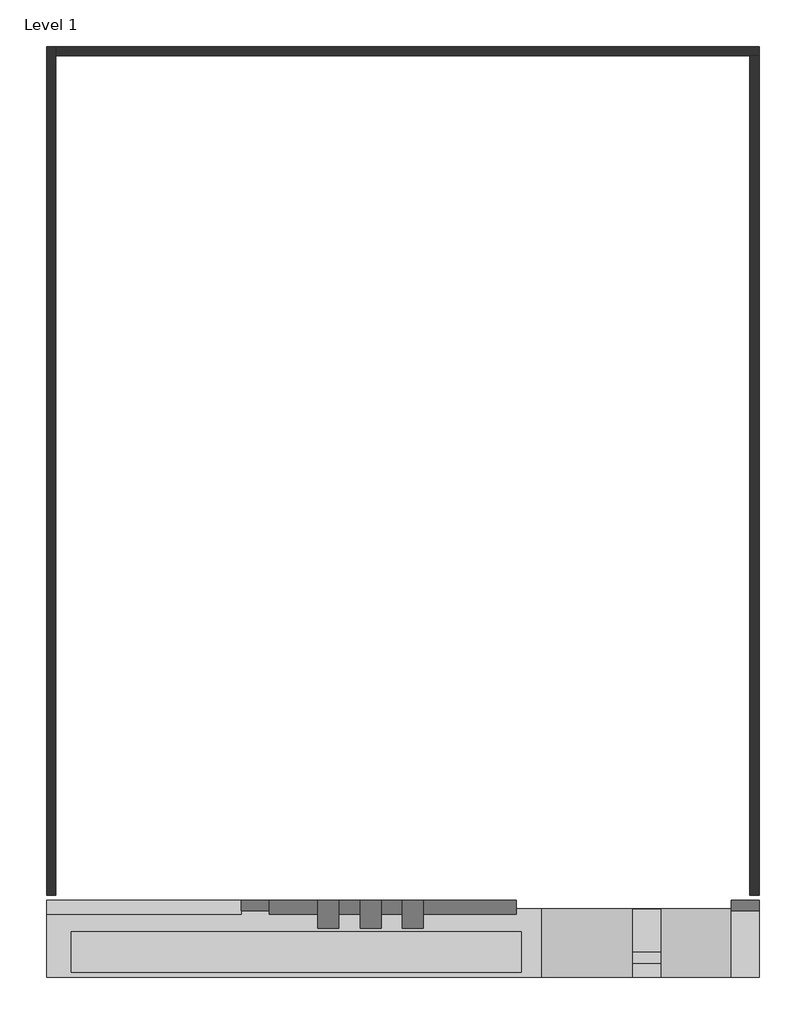
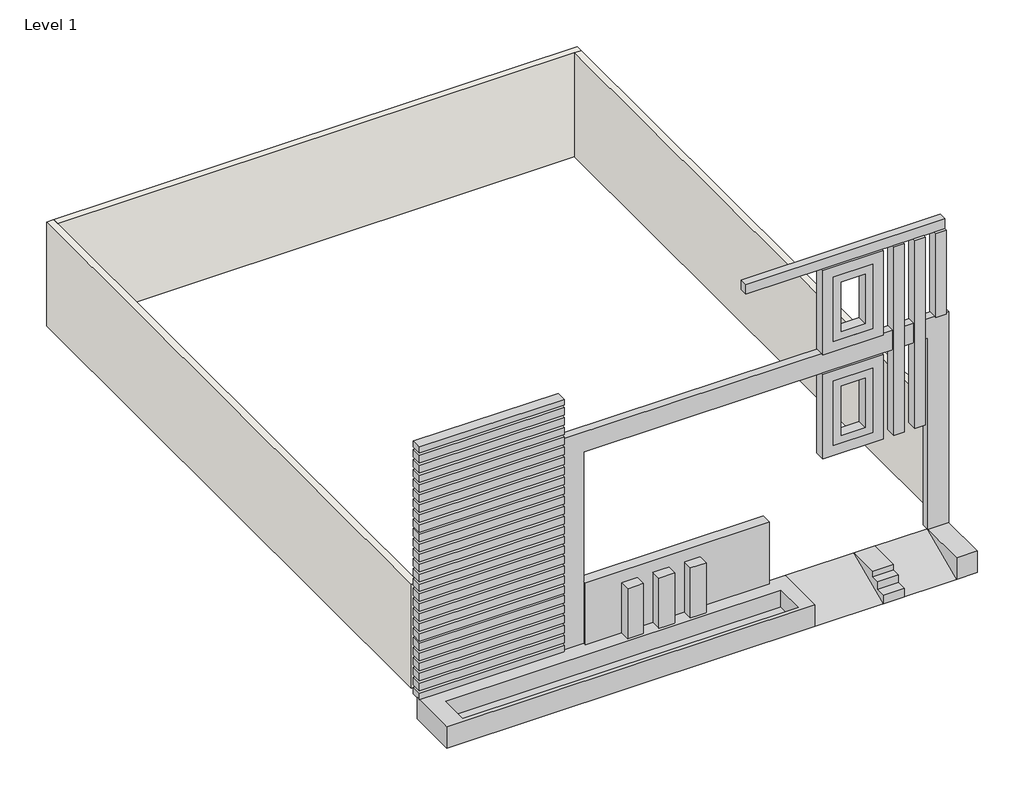
# One storey: 3 walls, 1 proxy.
"""IFC4 building model written with IfcOpenShell, lengths in millimetres."""

from ifc_helpers import new_model, si_unit, frame, origin, place, context, project, spatial, polyline, outline, extrude, faceted_brep, transform, mapped, element, save
from components import electrical_fixtures_1_electrical_fixtures_1_7c594ec0

model = new_model("IFC4")

# Units and contexts
model_context = context("Model", 3, world=origin())
ifc_project = project(units=[si_unit("LENGTHUNIT", "METRE", prefix="MILLI")], contexts=[model_context])

# Site, building, storey
site = spatial("IfcSite", under=ifc_project)
building = spatial("IfcBuilding", under=site)
storey = spatial("IfcBuildingStorey", under=building, Name="Level 1", Elevation=0.0)

# Proxy
placement = place(None, origin())
electrical_fixtures_1_electrical_fixtures_1_shape = electrical_fixtures_1_electrical_fixtures_1_7c594ec0(model_context)
element("IfcBuildingElementProxy", 1, Name="Electrical Fixtures 1 : Electrical Fixtures 1", ObjectType="Electrical Fixtures 1 : Electrical Fixtures 1", at=placement, inside=storey, context=model_context, shape_type="MappedRepresentation", body=[
    mapped(electrical_fixtures_1_electrical_fixtures_1_shape, transform((0.0, 0.0, 0.0), x_axis=(1.0, 0.0, 0.0), y_axis=(0.0, 1.0, 0.0), z_axis=(0.0, 0.0, 1.0))),
])

# Walls
element("IfcWall", 2, ObjectType="Generic - 8\"", at=placement, inside=storey, context=model_context, shape_type="SweptSolid", body=[
    extrude(outline(polyline([(7988.4813124, 3237.6669045), (7988.4813124, -14948.7330955), (7785.2813124, -14948.7330955), (7785.2813124, 3237.6669045), (7988.4813124, 3237.6669045)])), frame((0.0, 0.0, 762.0), z_axis=(0.0, 0.0, 1.0), x_axis=(1.0, 0.0, 0.0)), (0.0, 0.0, 1.0), 3200.4),
])
element("IfcWall", 3, ObjectType="Generic - 8\"", at=placement, inside=storey, context=model_context, shape_type="Brep", body=[
    faceted_brep([(7988.4813124, 3440.8669045, 762.0), (-7251.5186876, 3440.8669045, 762.0), (-7251.5186876, 3440.8669045, 3962.4), (7988.4813124, 3440.8669045, 3962.4), (7988.4813124, 3237.6669045, 762.0), (7988.4813124, 3237.6669045, 3962.4), (7785.2813124, 3237.6669045, 3962.4), (-7251.5186876, 3237.6669045, 3962.4), (-7251.5186876, 3237.6669045, 762.0), (7785.2813124, 3237.6669045, 762.0)], [[[0, 1, 2, 3]], [[4, 5, 6, 7, 8, 9]], [[1, 0, 4, 9, 8]], [[3, 2, 7, 6, 5]], [[2, 1, 8, 7]], [[0, 3, 5, 4]]]),
])
element("IfcWall", 4, ObjectType="Generic - 8\"", at=placement, inside=storey, context=model_context, shape_type="Brep", body=[
    faceted_brep([(-7454.7186876, 3440.8669045, 762.0), (-7454.7186876, -14948.7330955, 762.0), (-7454.7186876, -14948.7330955, 3962.4), (-7454.7186876, 3440.8669045, 3962.4), (-7251.5186876, 3440.8669045, 762.0), (-7251.5186876, 3440.8669045, 3962.4), (-7251.5186876, 3237.6669045, 3962.4), (-7251.5186876, -8179.6330955, 3962.4), (-7251.5186876, -8306.6330955, 3962.4), (-7251.5186876, -14948.7330955, 3962.4), (-7251.5186876, -14948.7330955, 762.0), (-7251.5186876, -8306.6330955, 762.0), (-7251.5186876, -8179.6330955, 762.0), (-7251.5186876, 3237.6669045, 762.0)], [[[0, 1, 2, 3]], [[4, 5, 6, 7, 8, 9, 10, 11, 12, 13]], [[0, 3, 5, 4]], [[1, 0, 4, 13, 12, 11, 10]], [[2, 1, 10, 9]], [[3, 2, 9, 8, 7, 6, 5]]]),
])

save(model, "model.ifc")

# Revit data of these elements
# Type "Generic - 8\""
#   Assembly Code = "B2010"
#   Layers, outside or top first: 0' - 8" no material (function 1)
# Element 1 (IfcBuildingElementProxy, "Electrical Fixtures 1 : Electrical Fixtures 1")
#   Mark = "1"
#   Phase Created = New Construction
#   Materials on its faces: "brown", "Concrete, Precast", "black"
# Elements 2, 3 (IfcWall, "Generic - 8\"")
#   built-in parameter 1001111 = 2' - 6"
#   Top Offset = 10' - 6"
#   Base Offset = 2' - 6"
#   wall height = 10' - 6"
#   Phase Created = New Construction
#   Base Constraint = Level 1
#   Top Constraint = Level 2
#   Materials on its faces: "Default Wall", "Clad - White"
# Element 4 (IfcWall, "Generic - 8\"")
#   built-in parameter 1001111 = 2' - 6"
#   Top Offset = 10' - 6"
#   Base Offset = 2' - 6"
#   wall height = 10' - 6"
#   Phase Created = New Construction
#   Base Constraint = Level 1
#   Top Constraint = Level 2
#   Materials on its faces: "Default Wall", "wall"
# Materials
#   "brown": class "Generic", colour RGB 89 45 45, transparency 0, Cost = 0
#   "Concrete, Precast": class "Concrete", colour RGB 198 187 187, transparency 0, Description = "Precast concrete", Cost = 0
#   "black": class "Generic", colour RGB 92 92 92, transparency 0, Cost = 0
#   "Default Wall": colour RGB 128 128 128, transparency 0, Cost = 0
#   "Clad - White": class "Wood", colour RGB 242 242 238, transparency 0, Cost = 0
#   "wall": class "Generic", colour RGB 255 0 128, transparency 0, Cost = 0
